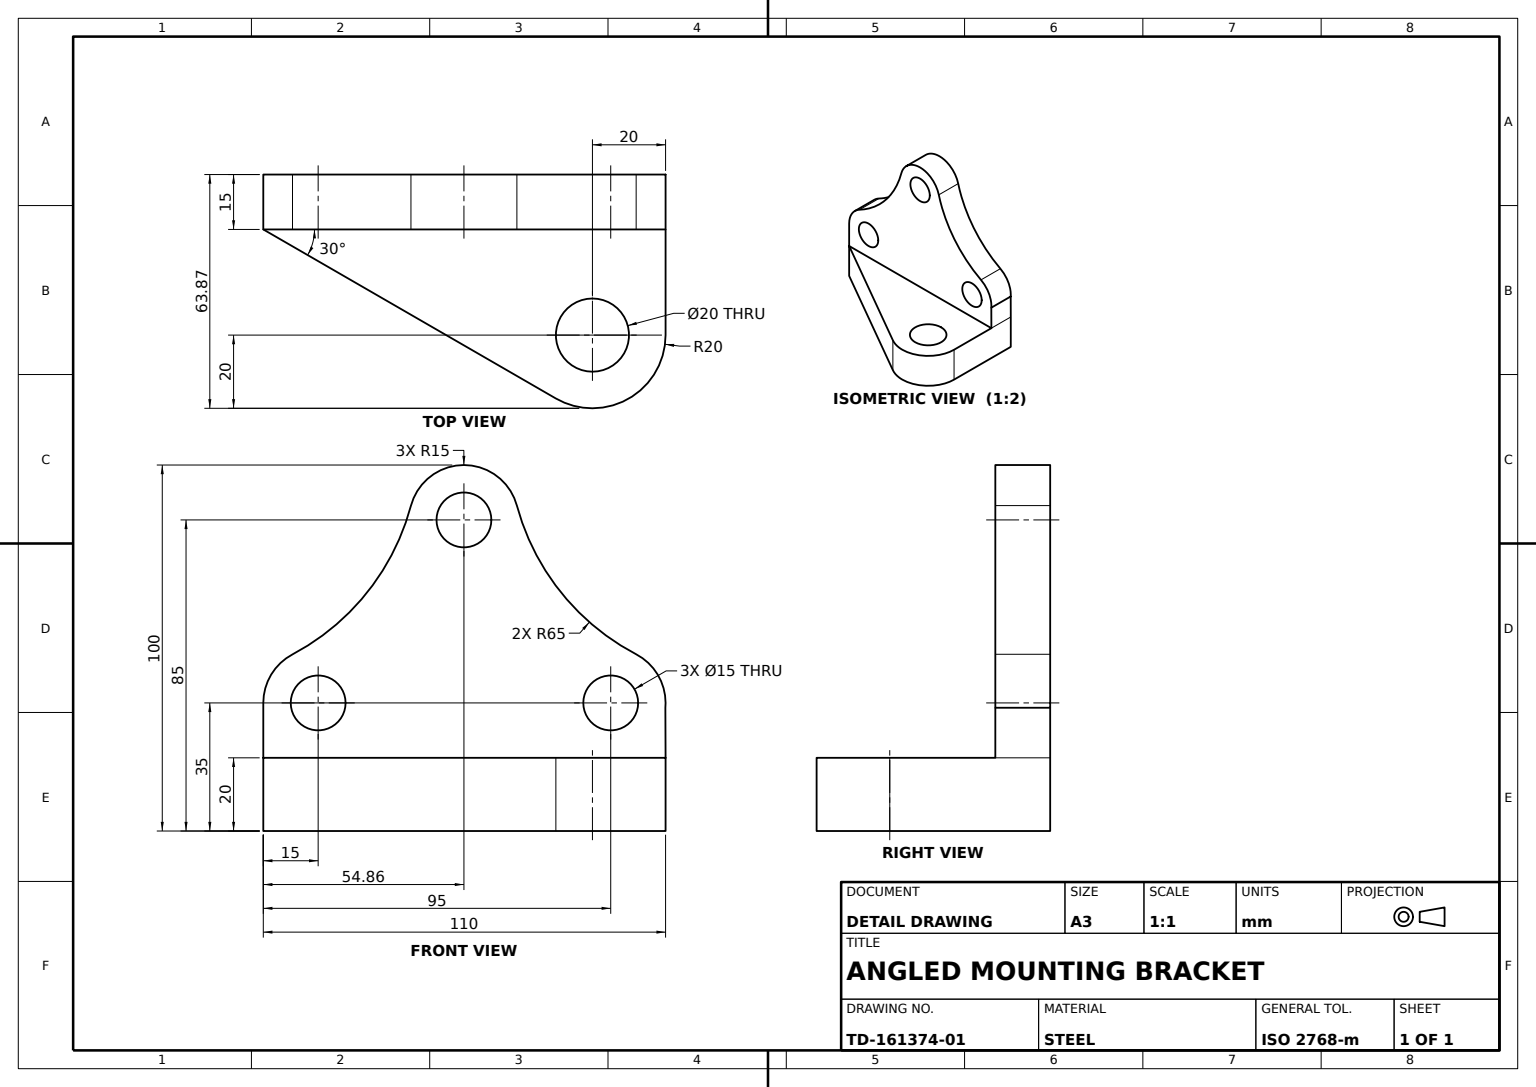
SolidWorks part; units mm, degrees
material "Plain Carbon Steel"
ref_plane "Front Plane" through (0, 0, 0) normal (0, 0, 1) x (1, 0, 0)
ref_plane "Top Plane" through (0, 0, 0) normal (0, 1, 0) x (1, 0, 0)
ref_plane "Right Plane" through (0, 0, 0) normal (1, 0, 0) x (0, 0, -1)
sketch "Base Wedge Profile Sketch" plane through (0, 0, 0) normal (0, 1, 0) x (1, 0, 0)
  line L0 (0, 0) -> (110, 0)
  line L1 (0, 0) -> (80, -46.188)
  line L2 (110, 0) -> (110, -28.8675)
  arc A0 (80, -46.188) -> (110, -28.8675) centre (90, -28.8675) ccw
  circle A1 centre (90, -28.8675) radius 10
  dimension "D2" = 20
  dimension "D4" = 20
  dimension "D1" = 30
  dimension "D3" = 110
extrude "Base Wedge Block" add sketch "Base Wedge Profile Sketch" against normal blind 20
sketch "Upright Flange Profile Sketch" plane through (0, 0, 0) normal (0, 0, -1) x (-1, 0, 0)
  line L0 (-55, 0) -> (-55, 112.1276) construction
  line L1 (-110, 0) -> (0, 0) construction
  line L2 (-109.9361, 15) -> (0, 15) construction
  line L3 (-95, 96.708) -> (-95, 2.451) construction
  line L4 (-15, 96.708) -> (-15, 2.451) construction
  line L5 (-110, 0) -> (-109.9417, 13.6788)
  line L6 (0, 15) -> (0, 0)
  line L7 (-110, 0) -> (0, 0)
  line L8 (-159.7234, 65) -> (50, 65) construction
  line L9 (0, -20) -> (-110, -20)
  line L10 (-159.9995, 0.2131) -> (-159.7234, 65) construction
  line L11 (50, 65) -> (50, 0) construction
  line L12 (-110, 0) -> (-109.9361, 15) construction
  line L13 (-110, -20) -> (-110, 0)
  circle A0 centre (-95, 15) radius 7.5
  arc A1 (-101.954, 28.2907) -> (-109.9417, 13.6788) centre (-95, 15) ccw
  circle A2 centre (-15, 15) radius 7.5
  arc A3 (0, 15) -> (-7.9856, 28.2589) centre (-15, 15) ccw
  arc A4 (-40.3733, 68.8839) -> (-69.3416, 68.9157) centre (-54.8617, 65) ccw
  circle A5 centre (-54.8617, 65) radius 7.5
  arc A6 (-101.954, 28.2907) -> (-69.3416, 68.9157) centre (-132.0878, 85.8837) ccw
  arc A7 (-40.3733, 68.8839) -> (-7.9856, 28.2589) centre (22.41, 85.7141) ccw
  line M18 (0, 0) -> (-110, 0)
  line M19 (-110, 0) -> (-110, -20)
  line M20 (-110, -20) -> (0, -20)
  line M21 (0, -20) -> (0, 0)
  dimension "D3" = 15
  dimension "D4" = 30
  dimension "D6" = 15
  dimension "D7" = 30
  dimension "D9" = 65
  dimension "D10" = 65
  dimension "D1" = 15
  dimension "D2" = 40
  dimension "D8" = 65
  dimension "D5" = 68.9157
  dimension "D11" = 55.1383
  dimension "D12" = 40.6584
  dimension "D13" = 40.3733
  dimension "D14" = 1.3212
  dimension "D15" = 15.0001
extrude "Upright Flange with Holes" add sketch "Upright Flange Profile Sketch" along normal blind 15 contours A7 A4 A6 A1 L5 L6 A3 A5 A2 A0 M18 | M21 M18 M19 M20
